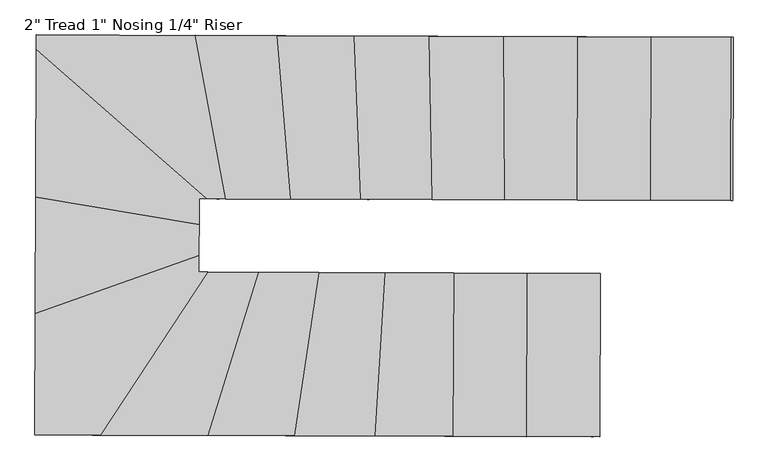
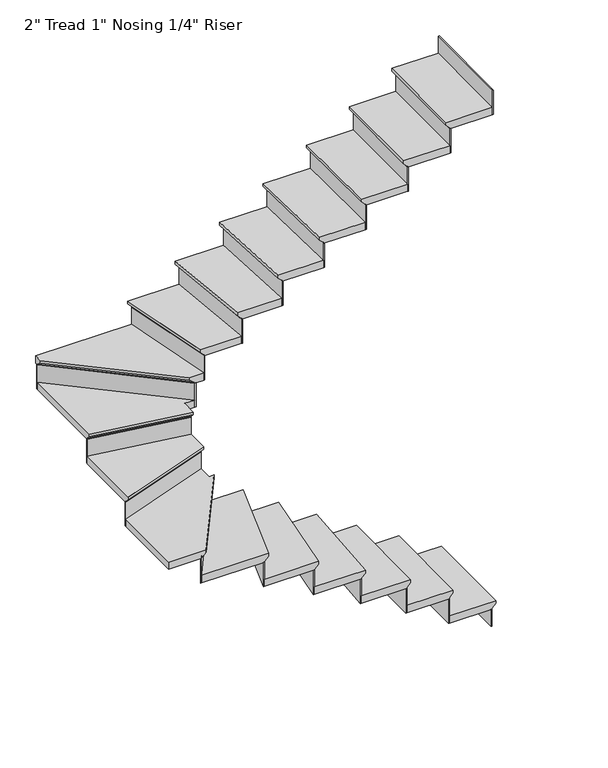
"""IFC4 building model written with IfcOpenShell, lengths in millimetres: stair flight geometry."""

from ifc_helpers import new_model, si_unit, origin, place, context, project, spatial, faceted_brep, source, transform, mapped, element, save


def stair_flight_765c7f0f(model_context):
    return source(origin(), model_context, "Body", "Brep", [
        faceted_brep([(-2339.9228929, -4204.0248458, 9751.4833333), (-2339.9228929, -4204.0248458, 9770.5333333), (-2342.0274141, -4826.0015756, 9770.5333333), (-2342.0274141, -4826.0015756, 9751.4833333), (-2365.3227475, -4203.9389029, 9726.0833333), (-2367.4272687, -4825.9156326, 9726.0833333), (-2644.7211481, -4202.9935301, 9770.5333333), (-2646.8256693, -4824.9702599, 9770.5333333), (-2367.4272687, -4825.9156326, 9719.7333333), (-2646.8256693, -4824.9702599, 9719.7333333), (-2644.7211481, -4202.9935301, 9719.7333333), (-2365.3227475, -4203.9389029, 9719.7333333)], [[[0, 1, 2, 3]], [[4, 0, 3, 5]], [[2, 1, 6, 7]], [[8, 9, 10, 11]], [[2, 7, 9, 8, 5, 3]], [[8, 11, 4, 5]], [[6, 1, 0, 4, 11, 10]], [[7, 6, 10, 9]]]),
        faceted_brep([(-2365.3227475, -4203.9389029, 9719.7333333), (-2365.3227475, -4203.9389029, 9601.2), (-2371.6727112, -4203.9174171, 9601.2), (-2371.6727112, -4203.9174171, 9719.7333333), (-2367.4272687, -4825.9156326, 9719.7333333), (-2373.7772323, -4825.8941469, 9719.7333333), (-2373.7772323, -4825.8941469, 9601.2), (-2367.4272687, -4825.9156326, 9601.2)], [[[0, 1, 2, 3]], [[4, 5, 6, 7]], [[1, 0, 4, 7]], [[2, 1, 7, 6]], [[3, 2, 6, 5]], [[0, 3, 5, 4]]]),
        faceted_brep([(-2644.7211481, -4202.9935301, 9889.0666667), (-2644.7211481, -4202.9935301, 9719.7333333), (-2651.0711118, -4202.9720444, 9719.7333333), (-2651.0711118, -4202.9720444, 9889.0666667), (-2646.8256693, -4824.9702599, 9889.0666667), (-2653.175633, -4824.9487741, 9889.0666667), (-2653.175633, -4824.9487741, 9719.7333333), (-2646.8256693, -4824.9702599, 9719.7333333)], [[[0, 1, 2, 3]], [[4, 5, 6, 7]], [[1, 0, 4, 7]], [[2, 1, 7, 6]], [[3, 2, 6, 5]], [[0, 3, 5, 4]]]),
        faceted_brep([(-2621.4258147, -4825.0562028, 9939.8666667), (-2619.3212935, -4203.0794731, 9939.8666667), (-2924.1195488, -4202.0481574, 9939.8666667), (-2926.2240699, -4824.0248871, 9939.8666667), (-2646.8256693, -4824.9702599, 9889.0666667), (-2926.2240699, -4824.0248871, 9889.0666667), (-2924.1195488, -4202.0481574, 9889.0666667), (-2644.7211481, -4202.9935301, 9889.0666667), (-2646.8256693, -4824.9702599, 9895.4166667), (-2621.4258147, -4825.0562028, 9920.8166667), (-2644.7211481, -4202.9935301, 9895.4166667), (-2619.3212935, -4203.0794731, 9920.8166667)], [[[0, 1, 2, 3]], [[4, 5, 6, 7]], [[0, 3, 5, 4, 8, 9]], [[4, 7, 10, 8]], [[2, 1, 11, 10, 7, 6]], [[3, 2, 6, 5]], [[11, 1, 0, 9]], [[10, 11, 9, 8]]]),
        faceted_brep([(-2924.1195488, -4202.0481574, 10058.4), (-2924.1195488, -4202.0481574, 9889.0666667), (-2930.4695124, -4202.0266716, 9889.0666667), (-2930.4695124, -4202.0266716, 10058.4), (-2926.2240699, -4824.0248871, 10058.4), (-2932.5740336, -4824.0034014, 10058.4), (-2932.5740336, -4824.0034014, 9889.0666667), (-2926.2240699, -4824.0248871, 9889.0666667)], [[[0, 1, 2, 3]], [[4, 5, 6, 7]], [[1, 0, 4, 7]], [[2, 1, 7, 6]], [[3, 2, 6, 5]], [[0, 3, 5, 4]]]),
        faceted_brep([(-2900.8242153, -4824.1108301, 10109.2), (-2898.7196941, -4202.1341003, 10109.2), (-3185.4282049, -4201.1639931, 10109.2), (-3223.7984946, -4823.0180139, 10109.2), (-2926.2240699, -4824.0248871, 10058.4), (-3223.7984946, -4823.0180139, 10058.4), (-3185.4282049, -4201.1639931, 10058.4), (-2924.1195488, -4202.0481574, 10058.4), (-2926.2240699, -4824.0248871, 10064.75), (-2900.8242153, -4824.1108301, 10090.15), (-2924.1195488, -4202.0481574, 10064.75), (-2898.7196941, -4202.1341003, 10090.15)], [[[0, 1, 2, 3]], [[4, 5, 6, 7]], [[0, 3, 5, 4, 8, 9]], [[4, 7, 10, 8]], [[2, 1, 11, 10, 7, 6]], [[3, 2, 6, 5]], [[11, 1, 0, 9]], [[10, 11, 9, 8]]]),
        faceted_brep([(-3185.4282049, -4201.1639931, 10227.7333333), (-3185.4282049, -4201.1639931, 10058.4), (-3191.7889535, -4201.1424708, 10058.4), (-3191.7889535, -4201.1424708, 10227.7333333), (-3223.7984946, -4823.0180139, 10227.7333333), (-3230.1592432, -4822.9964917, 10227.7333333), (-3230.1592432, -4822.9964917, 10058.4), (-3223.7984946, -4823.0180139, 10058.4)], [[[0, 1, 2, 3]], [[4, 5, 6, 7]], [[1, 0, 4, 7]], [[2, 1, 7, 6]], [[3, 2, 6, 5]], [[0, 3, 5, 4]]]),
        faceted_brep([(-3198.3555003, -4823.1041029, 10278.5333333), (-3159.9852105, -4201.250082, 10278.5333333), (-3437.1491731, -4200.3122697, 10278.5333333), (-3531.3418182, -4821.97741, 10278.5333333), (-3223.7984946, -4823.0180139, 10227.7333333), (-3531.3418182, -4821.97741, 10227.7333333), (-3437.1491731, -4200.3122697, 10227.7333333), (-3185.4282049, -4201.1639931, 10227.7333333), (-3223.7984946, -4823.0180139, 10234.0833333), (-3198.3555003, -4823.1041029, 10259.4833333), (-3185.4282049, -4201.1639931, 10234.0833333), (-3159.9852105, -4201.250082, 10259.4833333)], [[[0, 1, 2, 3]], [[4, 5, 6, 7]], [[0, 3, 5, 4, 8, 9]], [[4, 7, 10, 8]], [[2, 1, 11, 10, 7, 6]], [[3, 2, 6, 5]], [[11, 1, 0, 9]], [[10, 11, 9, 8]]]),
        faceted_brep([(-3437.1491731, -4200.3122697, 10397.0666667), (-3437.1491731, -4200.3122697, 10227.7333333), (-3443.568358, -4200.2905498, 10227.7333333), (-3443.568358, -4200.2905498, 10397.0666667), (-3531.3418182, -4821.97741, 10397.0666667), (-3537.7610031, -4821.95569, 10397.0666667), (-3537.7610031, -4821.95569, 10227.7333333), (-3531.3418182, -4821.97741, 10227.7333333)], [[[0, 1, 2, 3]], [[4, 5, 6, 7]], [[1, 0, 4, 7]], [[2, 1, 7, 6]], [[3, 2, 6, 5]], [[0, 3, 5, 4]]]),
        faceted_brep([(-3505.6650785, -4822.0642898, 10447.8666667), (-3411.4724335, -4200.3991496, 10447.8666667), (-3668.9000376, -4199.5281172, 10447.8666667), (-3860.1305452, -4820.8649201, 10447.8666667), (-3531.3418182, -4821.97741, 10397.0666667), (-3860.1305452, -4820.8649201, 10397.0666667), (-3668.9000376, -4199.5281172, 10397.0666667), (-3437.1491731, -4200.3122697, 10397.0666667), (-3531.3418182, -4821.97741, 10403.4166667), (-3505.6650785, -4822.0642898, 10428.8166667), (-3437.1491731, -4200.3122697, 10403.4166667), (-3411.4724335, -4200.3991496, 10428.8166667)], [[[0, 1, 2, 3]], [[4, 5, 6, 7]], [[0, 3, 5, 4, 8, 9]], [[4, 7, 10, 8]], [[2, 1, 11, 10, 7, 6]], [[3, 2, 6, 5]], [[11, 1, 0, 9]], [[10, 11, 9, 8]]]),
        faceted_brep([(-3668.9000376, -4199.5281172, 10566.4), (-3668.9000376, -4199.5281172, 10397.0666667), (-3675.5370713, -4199.5056601, 10397.0666667), (-3675.5370713, -4199.5056601, 10566.4), (-3860.1305452, -4820.8649201, 10566.4), (-3866.7675788, -4820.842463, 10566.4), (-3866.7675788, -4820.842463, 10397.0666667), (-3860.1305452, -4820.8649201, 10397.0666667)], [[[0, 1, 2, 3]], [[4, 5, 6, 7]], [[1, 0, 4, 7]], [[2, 1, 7, 6]], [[3, 2, 6, 5]], [[0, 3, 5, 4]]]),
        faceted_brep([(-3833.5824104, -4820.9547484, 10617.2), (-3642.3519028, -4199.6179455, 10617.2), (-3864.4957991, -4198.8662992, 10617.2), (-4274.0422035, -4819.4644081, 10617.2), (-3860.1305452, -4820.8649201, 10566.4), (-4274.0422035, -4819.4644081, 10566.4), (-3864.4957991, -4198.8662992, 10566.4), (-3668.9000376, -4199.5281172, 10566.4), (-3860.1305452, -4820.8649201, 10572.75), (-3833.5824104, -4820.9547484, 10598.15), (-3668.9000376, -4199.5281172, 10572.75), (-3642.3519028, -4199.6179455, 10598.15)], [[[0, 1, 2, 3]], [[4, 5, 6, 7]], [[0, 3, 5, 4, 8, 9]], [[4, 7, 10, 8]], [[2, 1, 11, 10, 7, 6]], [[3, 2, 6, 5]], [[11, 1, 0, 9]], [[10, 11, 9, 8]]]),
        faceted_brep([(-3864.4957991, -4198.8662992, 10735.7333333), (-3864.4957991, -4198.8662992, 10566.4), (-3872.0869257, -4198.8406138, 10566.4), (-3872.0869257, -4198.8406138, 10735.7333333), (-4274.0422035, -4819.4644081, 10735.7333333), (-4281.6333301, -4819.4387227, 10735.7333333), (-4281.6333301, -4819.4387227, 10566.4), (-4274.0422035, -4819.4644081, 10566.4)], [[[0, 1, 2, 3]], [[4, 5, 6, 7]], [[1, 0, 4, 7]], [[2, 1, 7, 6]], [[3, 2, 6, 5]], [[0, 3, 5, 4]]]),
        faceted_brep([(-4490.0684734, -4328.5349965, 10786.5333333), (-4491.7270905, -4818.7278493, 10786.5333333), (-4243.677697, -4819.5671495, 10786.5333333), (-3834.1312926, -4198.9690405, 10786.5333333), (-3867.6458395, -4198.8556407, 10786.5333333), (-3867.338948, -4108.1559559, 10786.5333333), (-4491.7270905, -4818.7278493, 10735.7333333), (-4490.0684734, -4328.5349965, 10735.7333333), (-3867.338948, -4108.1559559, 10735.7333333), (-3867.6458395, -4198.8556407, 10735.7333333), (-3864.4957991, -4198.8662992, 10735.7333333), (-4274.0422035, -4819.4644081, 10735.7333333), (-4274.0422035, -4819.4644081, 10742.0833333), (-4243.677697, -4819.5671495, 10767.4833333), (-3864.4957991, -4198.8662992, 10742.0833333), (-3834.1312926, -4198.9690405, 10767.4833333)], [[[0, 1, 2, 3, 4, 5]], [[6, 7, 8, 9, 10, 11]], [[1, 0, 7, 6]], [[2, 1, 6, 11, 12, 13]], [[11, 10, 14, 12]], [[4, 3, 15, 14, 10, 9]], [[5, 4, 9, 8]], [[0, 5, 8, 7]], [[15, 3, 2, 13]], [[14, 15, 13, 12]]]),
        faceted_brep([(-3867.338948, -4108.1559559, 10905.0666667), (-3867.338948, -4108.1559559, 10735.7333333), (-3867.316129, -4101.4119712, 10735.7333333), (-3867.316129, -4101.4119712, 10905.0666667), (-4490.0684734, -4328.5349965, 10905.0666667), (-4490.0456544, -4321.7910118, 10905.0666667), (-4490.0456544, -4321.7910118, 10735.7333333), (-4490.0684734, -4328.5349965, 10735.7333333)], [[[0, 1, 2, 3]], [[4, 5, 6, 7]], [[1, 0, 4, 7]], [[2, 1, 7, 6]], [[3, 2, 6, 5]], [[0, 3, 5, 4]]]),
        faceted_brep([(-4490.1597492, -4355.5109354, 10955.8666667), (-3867.4302238, -4135.1318948, 10955.8666667), (-3866.9449143, -3991.702012, 10955.8666667), (-4488.5718319, -3886.2129338, 10955.8666667), (-4490.0684734, -4328.5349965, 10905.0666667), (-4488.5718319, -3886.2129338, 10905.0666667), (-3866.9449143, -3991.702012, 10905.0666667), (-3867.338948, -4108.1559559, 10905.0666667), (-4490.0684734, -4328.5349965, 10911.4166667), (-4490.1597492, -4355.5109354, 10936.8166667), (-3867.338948, -4108.1559559, 10911.4166667), (-3867.4302238, -4135.1318948, 10936.8166667)], [[[0, 1, 2, 3]], [[4, 5, 6, 7]], [[0, 3, 5, 4, 8, 9]], [[4, 7, 10, 8]], [[3, 2, 6, 5]], [[11, 1, 0, 9]], [[10, 11, 9, 8]], [[2, 1, 11, 10, 7, 6]]]),
        faceted_brep([(-3866.9449143, -3991.702012, 11074.4), (-3866.9449143, -3991.702012, 10905.0666667), (-3866.9231337, -3985.2649249, 10905.0666667), (-3866.9231337, -3985.2649249, 11074.4), (-4488.5718319, -3886.2129338, 11074.4), (-4488.5500514, -3879.7758467, 11074.4), (-4488.5500514, -3879.7758467, 10905.0666667), (-4488.5718319, -3886.2129338, 10905.0666667)], [[[0, 1, 2, 3]], [[4, 5, 6, 7]], [[1, 0, 4, 7]], [[2, 1, 7, 6]], [[3, 2, 6, 5]], [[0, 3, 5, 4]]]),
        faceted_brep([(-4488.6589541, -3911.9612823, 11125.2), (-3867.0320364, -4017.4503605, 11125.2), (-3866.7004668, -3919.4572401, 11125.2), (-3799.1127501, -3919.6859299, 11125.2), (-4486.6423896, -3315.9795656, 11125.2), (-4488.5718319, -3886.2129338, 11074.4), (-4486.6423896, -3315.9795656, 11074.4), (-3799.1127501, -3919.6859299, 11074.4), (-3866.7004668, -3919.4572401, 11074.4), (-3866.9449143, -3991.702012, 11074.4), (-4488.5718319, -3886.2129338, 11080.75), (-4488.6589541, -3911.9612823, 11106.15), (-3866.9449143, -3991.702012, 11080.75), (-3867.0320364, -4017.4503605, 11106.15)], [[[0, 1, 2, 3, 4]], [[5, 6, 7, 8, 9]], [[0, 4, 6, 5, 10, 11]], [[5, 9, 12, 10]], [[2, 1, 13, 12, 9, 8]], [[4, 3, 7, 6]], [[13, 1, 0, 11]], [[12, 13, 11, 10]], [[3, 2, 8, 7]]]),
        faceted_brep([(-3799.1127501, -3919.6859299, 11243.7333333), (-3799.1127501, -3919.6859299, 11074.4), (-3789.4516067, -3919.7186194, 11074.4), (-3789.4516067, -3919.7186194, 11243.7333333), (-4486.6423896, -3315.9795656, 11243.7333333), (-4486.613881, -3307.5540264, 11243.7333333), (-4486.613881, -3307.5540264, 11074.4), (-4486.6423896, -3315.9795656, 11074.4)], [[[0, 1, 2, 3]], [[4, 5, 6, 7]], [[1, 0, 4, 7]], [[2, 1, 7, 6]], [[3, 2, 6, 5]], [[0, 3, 5, 4]]]),
        faceted_brep([(-3855.3688773, -3297.511731, 11294.5333333), (-4486.5726753, -3295.3759891, 11294.5333333), (-4486.7564243, -3349.6817226, 11294.5333333), (-3837.757324, -3919.5551721, 11294.5333333), (-3739.9081193, -3919.8862548, 11294.5333333), (-4486.5726753, -3295.3759891, 11243.7333333), (-3855.3688773, -3297.511731, 11243.7333333), (-3739.9081193, -3919.8862548, 11243.7333333), (-3799.1127501, -3919.6859299, 11243.7333333), (-4486.6423896, -3315.9795656, 11243.7333333), (-3799.1127501, -3919.6859299, 11250.0833333), (-4486.6423896, -3315.9795656, 11250.0833333), (-3837.757324, -3919.5551721, 11275.4833333), (-4486.7564243, -3349.6817226, 11275.4833333)], [[[0, 1, 2, 3, 4]], [[5, 6, 7, 8, 9]], [[1, 0, 6, 5]], [[9, 8, 10, 11]], [[4, 3, 12, 10, 8, 7]], [[0, 4, 7, 6]], [[12, 3, 2, 13]], [[10, 12, 13, 11]], [[2, 1, 5, 9, 11, 13]]]),
        faceted_brep([(-3739.9081193, -3919.8862548, 11413.0666667), (-3739.9081193, -3919.8862548, 11243.7333333), (-3733.4457151, -3919.908121, 11243.7333333), (-3733.4457151, -3919.908121, 11413.0666667), (-3855.3688773, -3297.511731, 11413.0666667), (-3848.9064731, -3297.5335972, 11413.0666667), (-3848.9064731, -3297.5335972, 11243.7333333), (-3855.3688773, -3297.511731, 11243.7333333)], [[[0, 1, 2, 3]], [[4, 5, 6, 7]], [[1, 0, 4, 7]], [[2, 1, 7, 6]], [[3, 2, 6, 5]], [[0, 3, 5, 4]]]),
        faceted_brep([(-3881.2184941, -3297.4242662, 11463.8666667), (-3765.7577361, -3919.79879, 11463.8666667), (-3493.4024921, -3920.7203315, 11463.8666667), (-3543.7965904, -3298.5659674, 11463.8666667), (-3855.3688773, -3297.511731, 11413.0666667), (-3543.7965904, -3298.5659674, 11413.0666667), (-3493.4024921, -3920.7203315, 11413.0666667), (-3739.9081193, -3919.8862548, 11413.0666667), (-3855.3688773, -3297.511731, 11419.4166667), (-3881.2184941, -3297.4242662, 11444.8166667), (-3739.9081193, -3919.8862548, 11419.4166667), (-3765.7577361, -3919.79879, 11444.8166667)], [[[0, 1, 2, 3]], [[4, 5, 6, 7]], [[0, 3, 5, 4, 8, 9]], [[4, 7, 10, 8]], [[2, 1, 11, 10, 7, 6]], [[3, 2, 6, 5]], [[11, 1, 0, 9]], [[10, 11, 9, 8]]]),
        faceted_brep([(-3493.4024921, -3920.7203315, 11582.4), (-3493.4024921, -3920.7203315, 11413.0666667), (-3487.0299488, -3920.7418937, 11413.0666667), (-3487.0299488, -3920.7418937, 11582.4), (-3543.7965904, -3298.5659674, 11582.4), (-3537.4240471, -3298.5875295, 11582.4), (-3537.4240471, -3298.5875295, 11413.0666667), (-3543.7965904, -3298.5659674, 11413.0666667)], [[[0, 1, 2, 3]], [[4, 5, 6, 7]], [[1, 0, 4, 7]], [[2, 1, 7, 6]], [[3, 2, 6, 5]], [[0, 3, 5, 4]]]),
        faceted_brep([(-3569.2867636, -3298.4797188, 11633.2), (-3518.8926653, -3920.634083, 11633.2), (-3226.664936, -3921.622865, 11633.2), (-3251.8690415, -3299.5537338, 11633.2), (-3543.7965904, -3298.5659674, 11582.4), (-3251.8690415, -3299.5537338, 11582.4), (-3226.664936, -3921.622865, 11582.4), (-3493.4024921, -3920.7203315, 11582.4), (-3543.7965904, -3298.5659674, 11588.75), (-3569.2867636, -3298.4797188, 11614.15), (-3493.4024921, -3920.7203315, 11588.75), (-3518.8926653, -3920.634083, 11614.15)], [[[0, 1, 2, 3]], [[4, 5, 6, 7]], [[0, 3, 5, 4, 8, 9]], [[4, 7, 10, 8]], [[2, 1, 11, 10, 7, 6]], [[3, 2, 6, 5]], [[11, 1, 0, 9]], [[10, 11, 9, 8]]]),
        faceted_brep([(-3226.664936, -3921.622865, 11751.7333333), (-3226.664936, -3921.622865, 11582.4), (-3220.3088547, -3921.6443715, 11582.4), (-3220.3088547, -3921.6443715, 11751.7333333), (-3251.8690415, -3299.5537338, 11751.7333333), (-3245.5129602, -3299.5752402, 11751.7333333), (-3245.5129602, -3299.5752402, 11582.4), (-3251.8690415, -3299.5537338, 11582.4)], [[[0, 1, 2, 3]], [[4, 5, 6, 7]], [[1, 0, 4, 7]], [[2, 1, 7, 6]], [[3, 2, 6, 5]], [[0, 3, 5, 4]]]),
        faceted_brep([(-3277.2933666, -3299.467708, 11802.5333333), (-3252.0892611, -3921.5368393, 11802.5333333), (-2953.9711928, -3922.5455519, 11802.5333333), (-2965.8021755, -3300.52167, 11802.5333333), (-3251.8690415, -3299.5537338, 11751.7333333), (-2965.8021755, -3300.52167, 11751.7333333), (-2953.9711928, -3922.5455519, 11751.7333333), (-3226.664936, -3921.622865, 11751.7333333), (-3251.8690415, -3299.5537338, 11758.0833333), (-3277.2933666, -3299.467708, 11783.4833333), (-3226.664936, -3921.622865, 11758.0833333), (-3252.0892611, -3921.5368393, 11783.4833333)], [[[0, 1, 2, 3]], [[4, 5, 6, 7]], [[0, 3, 5, 4, 8, 9]], [[4, 7, 10, 8]], [[2, 1, 11, 10, 7, 6]], [[3, 2, 6, 5]], [[11, 1, 0, 9]], [[10, 11, 9, 8]]]),
        faceted_brep([(-2953.9711928, -3922.5455519, 11921.0666667), (-2953.9711928, -3922.5455519, 11751.7333333), (-2947.6196355, -3922.567043, 11751.7333333), (-2947.6196355, -3922.567043, 11921.0666667), (-2965.8021755, -3300.52167, 11921.0666667), (-2959.4506182, -3300.5431611, 11921.0666667), (-2959.4506182, -3300.5431611, 11751.7333333), (-2965.8021755, -3300.52167, 11751.7333333)], [[[0, 1, 2, 3]], [[4, 5, 6, 7]], [[1, 0, 4, 7]], [[2, 1, 7, 6]], [[3, 2, 6, 5]], [[0, 3, 5, 4]]]),
        faceted_brep([(-2991.2084046, -3300.4357054, 11971.8666667), (-2979.3774219, -3922.4595874, 11971.8666667), (-2678.7239035, -3923.476879, 11971.8666667), (-2682.2633211, -3301.4810524, 11971.8666667), (-2965.8021755, -3300.52167, 11921.0666667), (-2682.2633211, -3301.4810524, 11921.0666667), (-2678.7239035, -3923.476879, 11921.0666667), (-2953.9711928, -3922.5455519, 11921.0666667), (-2965.8021755, -3300.52167, 11927.4166667), (-2991.2084046, -3300.4357054, 11952.8166667), (-2953.9711928, -3922.5455519, 11927.4166667), (-2979.3774219, -3922.4595874, 11952.8166667)], [[[0, 1, 2, 3]], [[4, 5, 6, 7]], [[0, 3, 5, 4, 8, 9]], [[4, 7, 10, 8]], [[2, 1, 11, 10, 7, 6]], [[3, 2, 6, 5]], [[11, 1, 0, 9]], [[10, 11, 9, 8]]]),
        faceted_brep([(-2678.7239035, -3923.476879, 12090.4), (-2678.7239035, -3923.476879, 11921.0666667), (-2672.3736784, -3923.4983656, 11921.0666667), (-2672.3736784, -3923.4983656, 12090.4), (-2682.2633211, -3301.4810524, 12090.4), (-2675.913096, -3301.502539, 12090.4), (-2675.913096, -3301.502539, 11921.0666667), (-2682.2633211, -3301.4810524, 11921.0666667)], [[[0, 1, 2, 3]], [[4, 5, 6, 7]], [[1, 0, 4, 7]], [[2, 1, 7, 6]], [[3, 2, 6, 5]], [[0, 3, 5, 4]]]),
        faceted_brep([(-2707.6642214, -3301.3951058, 12141.2), (-2704.1248038, -3923.3909324, 12141.2), (-2402.148518, -3924.4126998, 12141.2), (-2400.0439968, -3302.43597, 12141.2), (-2682.2633211, -3301.4810524, 12090.4), (-2400.0439968, -3302.43597, 12090.4), (-2402.148518, -3924.4126998, 12090.4), (-2678.7239035, -3923.476879, 12090.4), (-2682.2633211, -3301.4810524, 12096.75), (-2707.6642214, -3301.3951058, 12122.15), (-2678.7239035, -3923.476879, 12096.75), (-2704.1248038, -3923.3909324, 12122.15)], [[[0, 1, 2, 3]], [[4, 5, 6, 7]], [[0, 3, 5, 4, 8, 9]], [[4, 7, 10, 8]], [[2, 1, 11, 10, 7, 6]], [[3, 2, 6, 5]], [[11, 1, 0, 9]], [[10, 11, 9, 8]]]),
        faceted_brep([(-2402.148518, -3924.4126998, 12259.7333333), (-2402.148518, -3924.4126998, 12090.4), (-2395.7985543, -3924.4341855, 12090.4), (-2395.7985543, -3924.4341855, 12259.7333333), (-2400.0439968, -3302.43597, 12259.7333333), (-2393.6940331, -3302.4574557, 12259.7333333), (-2393.6940331, -3302.4574557, 12090.4), (-2400.0439968, -3302.43597, 12090.4)], [[[0, 1, 2, 3]], [[4, 5, 6, 7]], [[1, 0, 4, 7]], [[2, 1, 7, 6]], [[3, 2, 6, 5]], [[0, 3, 5, 4]]]),
        faceted_brep([(-2425.4438514, -3302.350027, 12310.5333333), (-2427.5483726, -3924.3267568, 12310.5333333), (-2122.7501174, -3925.3580725, 12310.5333333), (-2120.6455962, -3303.3813428, 12310.5333333), (-2400.0439968, -3302.43597, 12259.7333333), (-2120.6455962, -3303.3813428, 12259.7333333), (-2122.7501174, -3925.3580725, 12259.7333333), (-2402.148518, -3924.4126998, 12259.7333333), (-2400.0439968, -3302.43597, 12266.0833333), (-2425.4438514, -3302.350027, 12291.4833333), (-2402.148518, -3924.4126998, 12266.0833333), (-2427.5483726, -3924.3267568, 12291.4833333)], [[[0, 1, 2, 3]], [[4, 5, 6, 7]], [[0, 3, 5, 4, 8, 9]], [[4, 7, 10, 8]], [[2, 1, 11, 10, 7, 6]], [[3, 2, 6, 5]], [[11, 1, 0, 9]], [[10, 11, 9, 8]]]),
        faceted_brep([(-2122.7501174, -3925.3580725, 12429.0666667), (-2122.7501174, -3925.3580725, 12259.7333333), (-2116.4001537, -3925.3795583, 12259.7333333), (-2116.4001537, -3925.3795583, 12429.0666667), (-2120.6455962, -3303.3813428, 12429.0666667), (-2114.2956325, -3303.4028285, 12429.0666667), (-2114.2956325, -3303.4028285, 12259.7333333), (-2120.6455962, -3303.3813428, 12259.7333333)], [[[0, 1, 2, 3]], [[4, 5, 6, 7]], [[1, 0, 4, 7]], [[2, 1, 7, 6]], [[3, 2, 6, 5]], [[0, 3, 5, 4]]]),
        faceted_brep([(-1843.3517167, -3926.3034453, 12598.4), (-1843.3517167, -3926.3034453, 12429.0666667), (-1837.0017531, -3926.324931, 12429.0666667), (-1837.0017531, -3926.324931, 12598.4), (-1841.2471955, -3304.3267155, 12598.4), (-1834.8972319, -3304.3482013, 12598.4), (-1834.8972319, -3304.3482013, 12429.0666667), (-1841.2471955, -3304.3267155, 12429.0666667)], [[[0, 1, 2, 3]], [[4, 5, 6, 7]], [[1, 0, 4, 7]], [[2, 1, 7, 6]], [[3, 2, 6, 5]], [[0, 3, 5, 4]]]),
        faceted_brep([(-2146.0454508, -3303.2953998, 12479.8666667), (-2148.149972, -3925.2721295, 12479.8666667), (-1843.3517167, -3926.3034453, 12479.8666667), (-1841.2471955, -3304.3267155, 12479.8666667), (-2120.6455962, -3303.3813428, 12429.0666667), (-1841.2471955, -3304.3267155, 12429.0666667), (-1843.3517167, -3926.3034453, 12429.0666667), (-2122.7501174, -3925.3580725, 12429.0666667), (-2120.6455962, -3303.3813428, 12435.4166667), (-2146.0454508, -3303.2953998, 12460.8166667), (-2122.7501174, -3925.3580725, 12435.4166667), (-2148.149972, -3925.2721295, 12460.8166667)], [[[0, 1, 2, 3]], [[4, 5, 6, 7]], [[0, 3, 5, 4, 8, 9]], [[4, 7, 10, 8]], [[2, 1, 11, 10, 7, 6]], [[3, 2, 6, 5]], [[11, 1, 0, 9]], [[10, 11, 9, 8]]]),
    ])


if __name__ == "__main__":
    model = new_model("IFC4")
    model_context = context("Model", 3, world=origin())
    ifc_project = project(units=[si_unit("LENGTHUNIT", "METRE", prefix="MILLI")], contexts=[model_context])
    site = spatial("IfcSite", under=ifc_project)
    building = spatial("IfcBuilding", under=site)
    placement = place(None, origin())
    stair_flight_shape = stair_flight_765c7f0f(model_context)
    element("IfcStairFlight", 1, ObjectType="2\" Tread 1\" Nosing 1/4\" Riser", at=placement, inside=building, context=model_context, shape_type="MappedRepresentation", body=[
        mapped(stair_flight_shape, transform((0.0, 0.0, 0.0), x_axis=(1.0, 0.0, 0.0), y_axis=(0.0, 1.0, 0.0), z_axis=(0.0, 0.0, 1.0))),
    ])
    save(model, "model.ifc")
